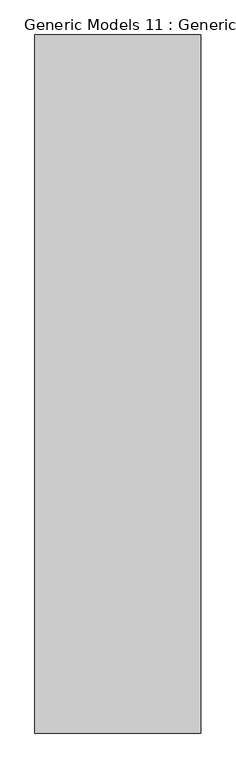
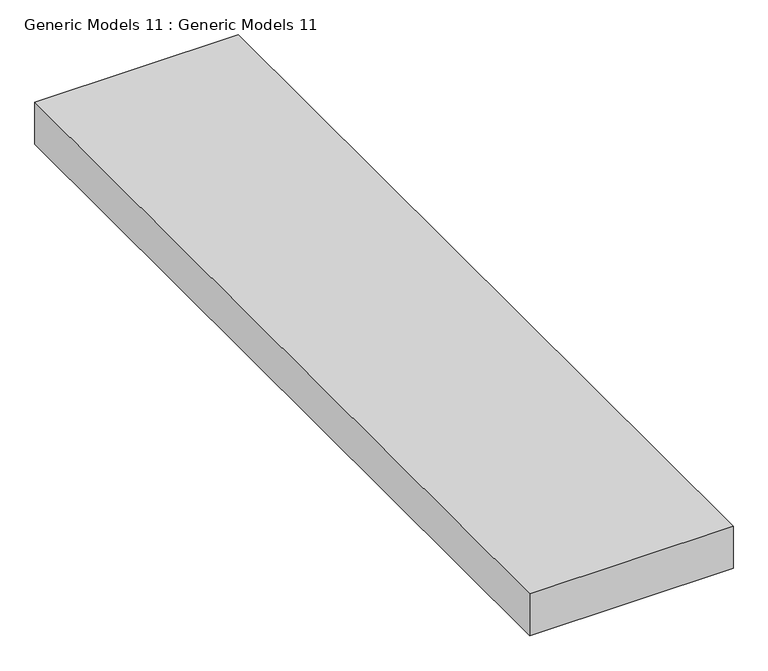
"""IFC4 building model written with IfcOpenShell, lengths in millimetres: proxy geometry, Generic Models 11 : Generic Models 11."""

from ifc_helpers import new_model, si_unit, frame, origin, place, context, project, spatial, polyline, outline, extrude, source, transform, mapped, element, save


def generic_models_11_generic_models_11_762d5f7a(model_context):
    return source(origin(), model_context, "Body", "SweptSolid", [
        extrude(outline(polyline([(-8497.9161422, -13389.119515), (-9196.4161422, -13389.119515), (-9196.4161422, -10446.5171312), (-8497.9161422, -10446.5171312), (-8497.9161422, -13389.119515)])), frame((0.0, 0.0, 5616.1380633), z_axis=(0.0, 0.0, 1.0), x_axis=(1.0, 0.0, 0.0)), (0.0, 0.0, 1.0), 152.4),
    ])


if __name__ == "__main__":
    model = new_model("IFC4")
    model_context = context("Model", 3, world=origin())
    ifc_project = project(units=[si_unit("LENGTHUNIT", "METRE", prefix="MILLI")], contexts=[model_context])
    site = spatial("IfcSite", under=ifc_project)
    building = spatial("IfcBuilding", under=site)
    placement = place(None, origin())
    generic_models_11_generic_models_11_shape = generic_models_11_generic_models_11_762d5f7a(model_context)
    element("IfcBuildingElementProxy", 1, Name="Generic Models 11 : Generic Models 11", ObjectType="Generic Models 11 : Generic Models 11", at=placement, inside=building, context=model_context, shape_type="MappedRepresentation", body=[
        mapped(generic_models_11_generic_models_11_shape, transform((0.0, 0.0, 0.0), x_axis=(1.0, 0.0, 0.0), y_axis=(0.0, 1.0, 0.0), z_axis=(0.0, 0.0, 1.0))),
    ])
    save(model, "model.ifc")
